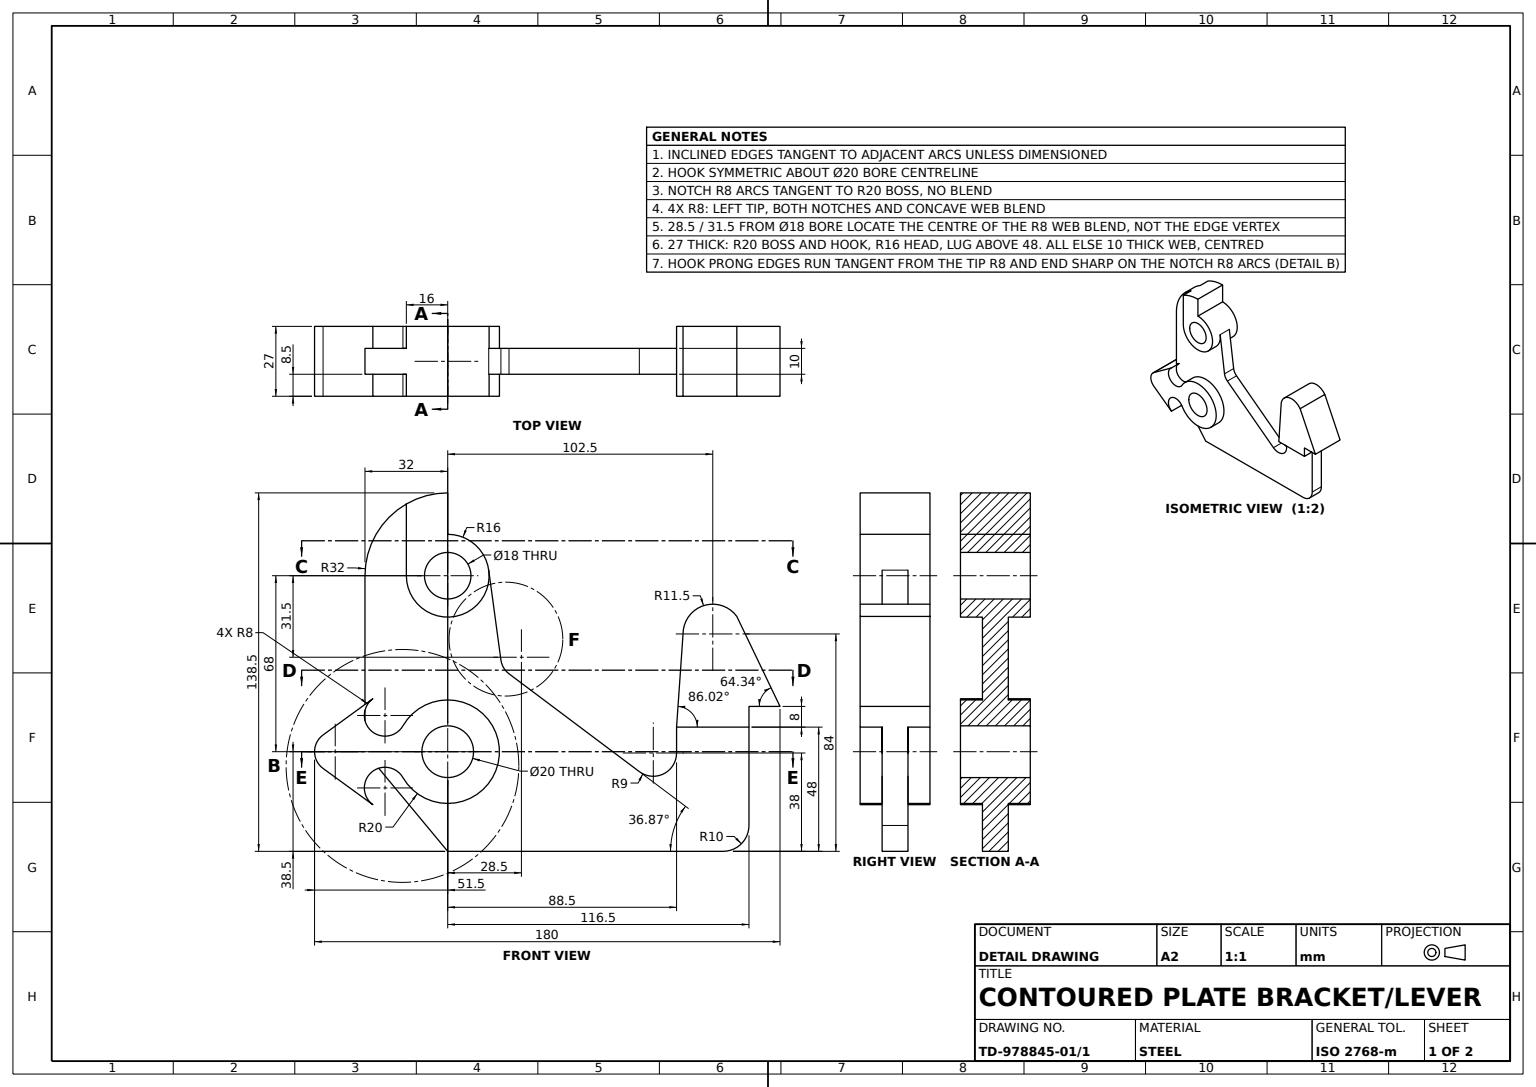
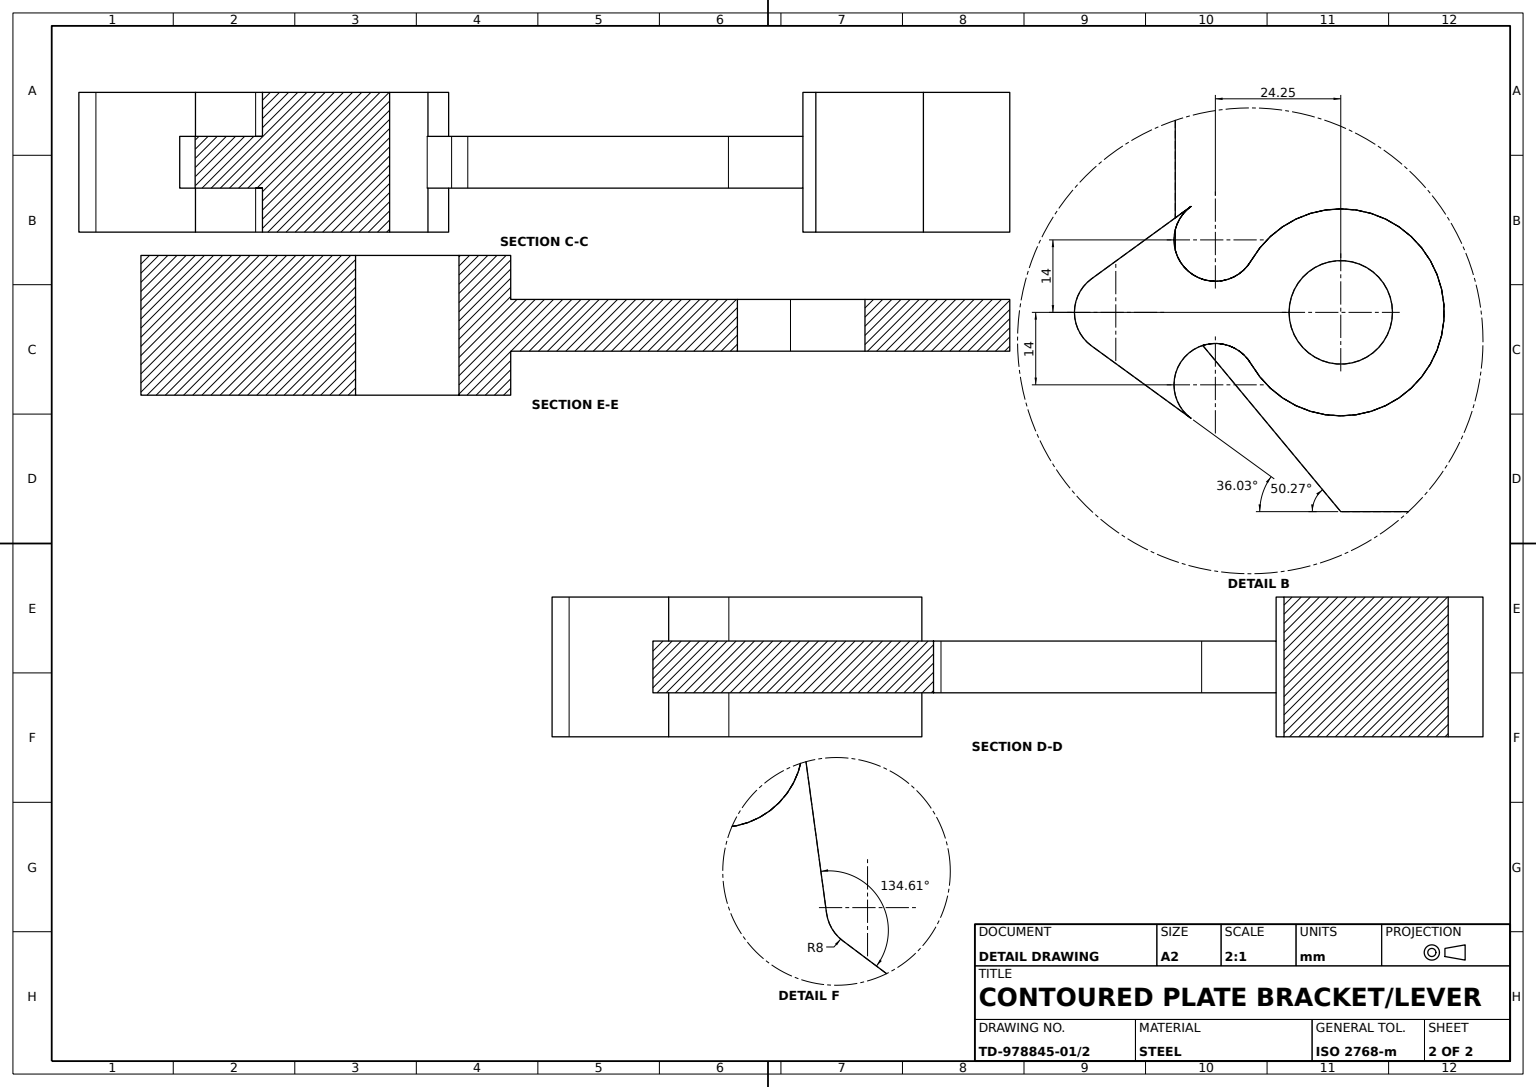
SolidWorks part; units mm, degrees
material "Plain Carbon Steel"
ref_plane "Front Plane" through (0, 0, 0) normal (0, 0, 1) x (1, 0, 0)
ref_plane "Top Plane" through (0, 0, 0) normal (0, 1, 0) x (1, 0, 0)
ref_plane "Right Plane" through (0, 0, 0) normal (1, 0, 0) x (0, 0, -1)
sketch "Bracket Plate Profile" plane through (0, 0, 0) normal (0, 0, 1) x (1, 0, 0)
  line L0 (-32, 0) -> (-32, -68)
  line L1 (-32, -68) -> (0, -106.5)
  line L2 (0, -106.5) -> (116.5, -106.5)
  line L3 (116.5, -106.5) -> (116.5, -58.5)
  line L4 (116.5, -58.5) -> (88.5, -58.5)
  line L5 (88.5, -58.5) -> (88.5, -68.5)
  line L6 (15.8544, 2.1539) -> (20.5728, -32.577)
  line L7 (23.7, -37.9) -> (74.1, -75.7)
  line L8 (0, 16) -> (0, 32)
  arc A0 (0, 32) -> (-32, 0) centre (0, 0) ccw
  arc A1 (74.1, -75.7) -> (88.5, -68.5) centre (79.5, -68.5) ccw
  arc A2 (20.5728, -32.577) -> (23.7, -37.9) centre (28.5, -31.5) ccw
  arc A3 (15.8544, 2.1539) -> (0, 16) centre (0, 0) ccw
  dimension "D1" = 64
  dimension "D3" = 18
  dimension "D6" = 16
  dimension "D9" = 32
  dimension "D2" = 38.5
  dimension "D4" = 37
  dimension "D5" = 38
  dimension "D7" = 75
  dimension "D8" = 88
  dimension "D10" = 116.5
  dimension "D11" = 50.0625
  dimension "D12" = 48
  dimension "D13" = 106.5
extrude "Bracket Plate" add sketch "Bracket Plate Profile" along normal blind 10
ref_plane "Boss Offset Plane" through (0, 0, 5) normal (0, 0, 1) x (1, 0, 0)
sketch "Upper Pivot Boss Profile" plane through (0, 0, 5) normal (0, 0, 1) x (1, 0, 0)
  line L0 (0, 16) -> (0, 32)
  line L1 (-16, 0) -> (-16, 27.7128)
  arc A0 (-16, 0) -> (0, 16) centre (0, 0) ccw
  arc A1 (0, 32) -> (-16, 27.7128) centre (0, 0) ccw
  dimension "D2" = 64
extrude "Upper Pivot Boss" add sketch "Upper Pivot Boss Profile" along normal mid plane 27
sketch "Upper Pivot Bore Profile" plane through (0, 0, 18.5) normal (0, 0, 1) x (1, 0, 0)
  circle A0 centre (0, 0) radius 9
  dimension "D1" = 18
extrude "Upper Pivot Bore Ø18" cut sketch "Upper Pivot Bore Profile" against normal blind 27
sketch "Lower Pivot Boss Profile" plane through (0, 0, 5) normal (0, 0, 1) x (1, 0, 0)
  line L0 (0, -106.5) -> (116.5, -106.5) construction
  line L1 (-32, 0) -> (-32, -68) construction
  line L2 (-48.2052, -74.47) -> (-28.9539, -88.47)
  line L3 (-48.2052, -61.53) -> (-28.9539, -47.53)
  arc A0 (-17.3205, -78) -> (-17.3205, -58) centre (0, -68) ccw
  arc A1 (-48.2052, -61.53) -> (-48.2052, -74.47) centre (-43.5, -68) ccw
  arc A2 (-28.9539, -47.53) -> (-17.3205, -58) centre (-24.2487, -54) ccw
  arc A3 (-17.3205, -78) -> (-28.9539, -88.47) centre (-24.2487, -82) ccw
  dimension "D1" = 40
  dimension "D6" = 16
  dimension "D7" = 16
  dimension "D8" = 16
  dimension "D2" = 38.5
  dimension "D3" = 32
  dimension "D4" = 43.5
  dimension "D5" = 68
  dimension "D9" = 24.2487
  dimension "D10" = 54
extrude "Lower Pivot Boss" add sketch "Lower Pivot Boss Profile" along normal mid plane 27
sketch "Lower Pivot Bore Profile" plane through (0, 0, 18.5) normal (0, 0, 1) x (1, 0, 0)
  circle A0 centre (0, -68) radius 10
  dimension "D1" = 20
extrude "Lower Pivot Bore Ø20" cut sketch "Lower Pivot Bore Profile" against normal blind 27
sketch "Stop Lug Profile" plane through (0, 0, 5) normal (0, 0, 1) x (1, 0, 0)
  line L0 (0, -106.5) -> (116.5, -106.5) construction
  line L1 (116.5, -58.5) -> (116.5, -50.5)
  line L2 (116.5, -50.5) -> (128.5, -50.5)
  line L3 (128.5, -50.5) -> (111.7974, -15.7318)
  line L4 (91, -22.5) -> (88.5, -58.5)
  line L6 (88.5, -58.5) -> (116.5, -58.5)
  arc A0 (111.7974, -15.7318) -> (91, -22.5) centre (102.5, -22.5) ccw
  dimension "D1" = 23
  dimension "D2" = 84
  dimension "D3" = 102.5
  dimension "D4" = 8
  dimension "D5" = 12
  dimension "D6" = 38.5721
extrude "Stop Lug" add sketch "Stop Lug Profile" along normal mid plane 27
fillet "Plate Fillet R10" radius 10 1 edges at (116.5, -106.5, 5)
